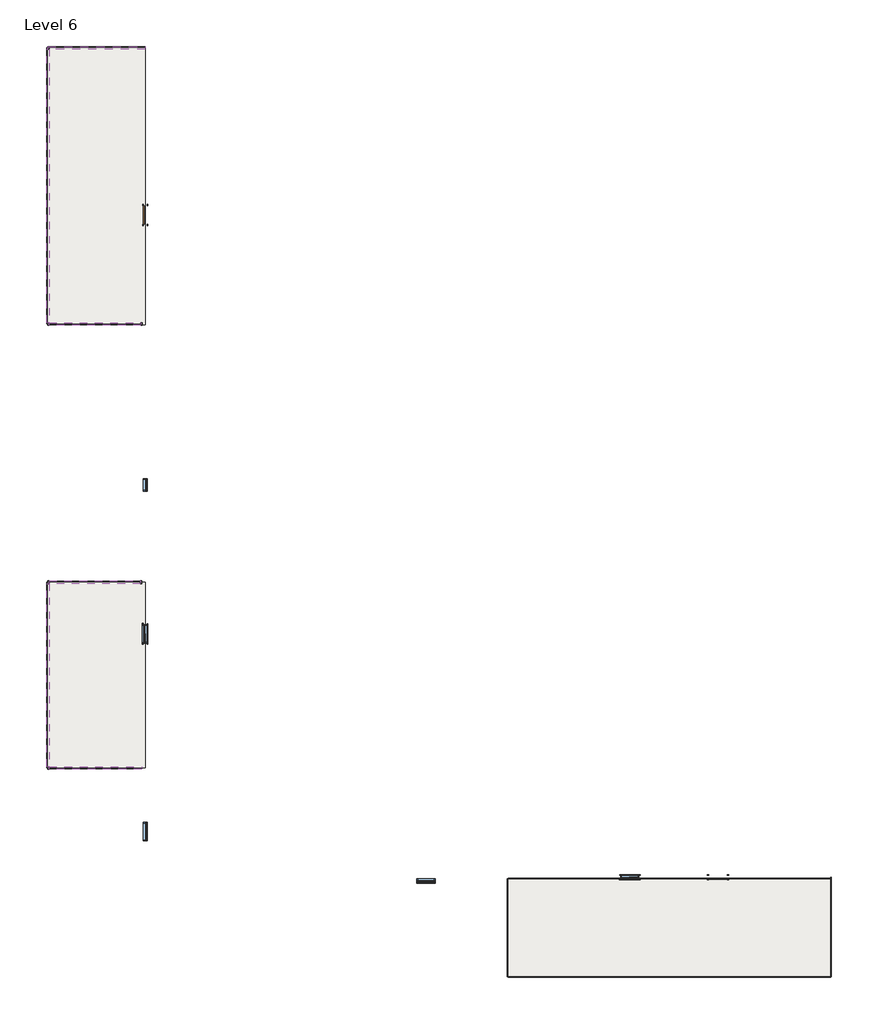
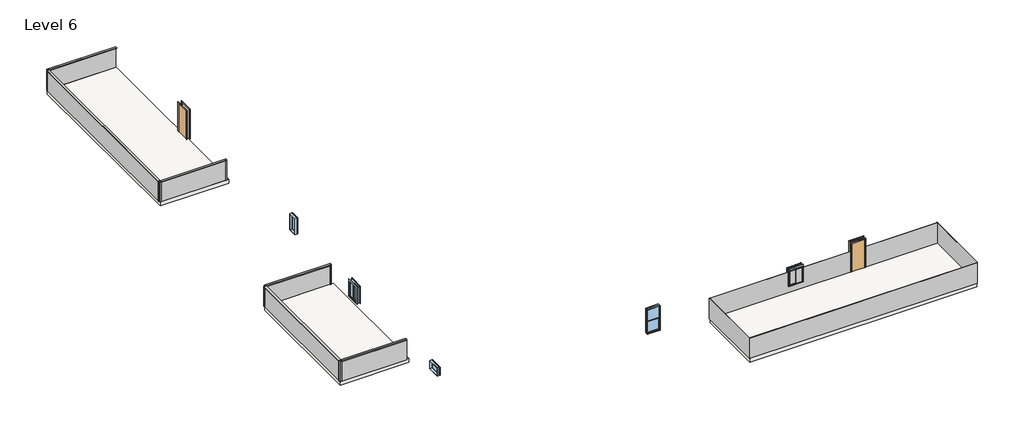
# One storey: 15 members, 10 plates, 5 windows, 3 slabs, 2 doors.
"""IFC4 building model written with IfcOpenShell, lengths in millimetres."""

from ifc_helpers import new_model, si_unit, frame, origin, place, context, project, spatial, polyline, outline, extrude, transform, mapped, element, save
from components import door_54dd4da4, door_719f80de, member_4491d118, member_b978f1c8, member_fc9bce7c, member_8787ee90, member_f500ba6f, member_67196db4, member_44cf4dfe, system_panel_glazed_dbf8c7ac, system_panel_glazed_64af9de3, system_panel_glazed_abcfc967, system_panel_glazed_6e908680, system_panel_glazed_242742f8, system_panel_glazed_fce9463a, system_panel_glazed_c13b8b16, system_panel_glazed_066de0f8, system_panel_glazed_7f285cc4, window_f274a882, window_80bd9af0, window_57c3ee1c, window_54100e87

model = new_model("IFC4")

# Units and contexts
model_context = context("Model", 3, world=origin())
ifc_project = project(units=[si_unit("LENGTHUNIT", "METRE", prefix="MILLI")], contexts=[model_context])

# Site, building, storey
site = spatial("IfcSite", under=ifc_project)
building = spatial("IfcBuilding", under=site)
storey = spatial("IfcBuildingStorey", under=building, Name="Level 6", Elevation=9753.6)

# Doors
placement = place(None, origin())
door_shape = door_54dd4da4(model_context)
element("IfcDoor", 1, ObjectType="Single-Flush : 36\" x 84\"", at=placement, inside=storey, context=model_context, shape_type="MappedRepresentation", body=[
    mapped(door_shape, transform((-15175.038074, 12428.2014639, 9753.6), x_axis=(0.0, 1.0, 0.0), y_axis=(-1.0, 0.0, 0.0), z_axis=(0.0, 0.0, 1.0))),
])
door_2_shape = door_719f80de(model_context)
element("IfcDoor", 2, ObjectType="Single-Flush : 36\" x 84\"", at=placement, inside=storey, context=model_context, shape_type="MappedRepresentation", body=[
    mapped(door_2_shape, transform((13526.961926, -20744.1985361, 9753.6), x_axis=(1.0, 0.0, 0.0), y_axis=(0.0, 1.0, 0.0), z_axis=(0.0, 0.0, 1.0))),
])

# Members
member_shape = member_4491d118(model_context)
element("IfcMember", 3, ObjectType="Rectangular Mullion : 2.5\" x 5\" rectangular", at=placement, inside=storey, context=model_context, shape_type="MappedRepresentation", body=[
    mapped(member_shape, transform((-20051.838074, 6979.9014639, 9753.6), x_axis=(-1.0, 0.0, 0.0), y_axis=(0.0, 1.0, 0.0), z_axis=(0.0, 0.0, -1.0))),
])
element("IfcMember", 4, ObjectType="Rectangular Mullion : 2.5\" x 5\" rectangular", at=placement, inside=storey, context=model_context, shape_type="MappedRepresentation", body=[
    mapped(member_shape, transform((-20051.838074, 20810.2014639, 9753.6), x_axis=(0.0, 1.0, 0.0), y_axis=(1.0, 0.0, 0.0), z_axis=(0.0, 0.0, -1.0))),
])
element("IfcMember", 5, ObjectType="Rectangular Mullion : 2.5\" x 5\" rectangular", at=placement, inside=storey, context=model_context, shape_type="MappedRepresentation", body=[
    mapped(member_shape, transform((-20051.838074, -5966.8213044, 9753.6), x_axis=(0.0, 1.0, 0.0), y_axis=(1.0, 0.0, 0.0), z_axis=(0.0, 0.0, -1.0))),
])
element("IfcMember", 6, ObjectType="Rectangular Mullion : 2.5\" x 5\" rectangular", at=placement, inside=storey, context=model_context, shape_type="MappedRepresentation", body=[
    mapped(member_shape, transform((-15357.6517659, -5966.8213044, 9753.6), x_axis=(1.0, 0.0, 0.0), y_axis=(0.0, -1.0, 0.0), z_axis=(0.0, 0.0, -1.0))),
])
element("IfcMember", 7, ObjectType="Rectangular Mullion : 2.5\" x 5\" rectangular", at=placement, inside=storey, context=model_context, shape_type="MappedRepresentation", body=[
    mapped(member_shape, transform((-20051.838074, -15263.2213044, 9753.6), x_axis=(-1.0, 0.0, 0.0), y_axis=(0.0, 1.0, 0.0), z_axis=(0.0, 0.0, -1.0))),
])
element("IfcMember", 8, ObjectType="Rectangular Mullion : 2.5\" x 5\" rectangular", at=placement, inside=storey, context=model_context, shape_type="MappedRepresentation", body=[
    mapped(member_shape, transform((-20051.838074, 6979.9014639, 11277.6), x_axis=(0.0, -1.0, 0.0), y_axis=(1.0, 0.0, 0.0), z_axis=(0.0, 0.0, 1.0))),
])
element("IfcMember", 9, ObjectType="Rectangular Mullion : 2.5\" x 5\" rectangular", at=placement, inside=storey, context=model_context, shape_type="MappedRepresentation", body=[
    mapped(member_shape, transform((-20051.838074, -5966.8213044, 11277.6), x_axis=(-1.0, 0.0, 0.0), y_axis=(0.0, -1.0, 0.0), z_axis=(0.0, 0.0, 1.0))),
])
element("IfcMember", 10, ObjectType="Rectangular Mullion : 2.5\" x 5\" rectangular", at=placement, inside=storey, context=model_context, shape_type="MappedRepresentation", body=[
    mapped(member_shape, transform((-20051.838074, -15263.2213044, 11277.6), x_axis=(0.0, -1.0, 0.0), y_axis=(1.0, 0.0, 0.0), z_axis=(0.0, 0.0, 1.0))),
])
element("IfcMember", 11, ObjectType="Rectangular Mullion : 2.5\" x 5\" rectangular", at=placement, inside=storey, context=model_context, shape_type="MappedRepresentation", body=[
    mapped(member_shape, transform((-15327.438074, 6979.9014639, 11277.6), x_axis=(1.0, 0.0, 0.0), y_axis=(0.0, 1.0, 0.0), z_axis=(0.0, 0.0, 1.0))),
])
member_2_shape = member_b978f1c8(model_context)
element("IfcMember", 12, ObjectType="Rectangular Mullion : 2.5\" x 5\" rectangular", at=placement, inside=storey, context=model_context, shape_type="MappedRepresentation", body=[
    mapped(member_2_shape, transform((-20051.838074, 20746.7014639, 11277.6), x_axis=(0.0, 0.0, 1.0), y_axis=(1.0, 0.0, 0.0), z_axis=(0.0, 1.0, 0.0))),
])
member_3_shape = member_fc9bce7c(model_context)
element("IfcMember", 13, ObjectType="Rectangular Mullion : 2.5\" x 5\" rectangular", at=placement, inside=storey, context=model_context, shape_type="MappedRepresentation", body=[
    mapped(member_3_shape, transform((-15175.038074, 20810.2014639, 11277.6), x_axis=(0.0, 0.0, 1.0), y_axis=(0.0, -1.0, 0.0), z_axis=(1.0, 0.0, 0.0))),
])
member_4_shape = member_8787ee90(model_context)
element("IfcMember", 14, ObjectType="Rectangular Mullion : 2.5\" x 5\" rectangular", at=placement, inside=storey, context=model_context, shape_type="MappedRepresentation", body=[
    mapped(member_4_shape, transform((-20051.838074, -6030.3213044, 11277.6), x_axis=(0.0, 0.0, 1.0), y_axis=(1.0, 0.0, 0.0), z_axis=(0.0, 1.0, 0.0))),
])
member_5_shape = member_f500ba6f(model_context)
element("IfcMember", 15, ObjectType="Rectangular Mullion : 2.5\" x 5\" rectangular", at=placement, inside=storey, context=model_context, shape_type="MappedRepresentation", body=[
    mapped(member_5_shape, transform((-15421.1517659, -5966.8213044, 11277.6), x_axis=(0.0, 0.0, 1.0), y_axis=(0.0, -1.0, 0.0), z_axis=(1.0, 0.0, 0.0))),
])
member_6_shape = member_67196db4(model_context)
element("IfcMember", 16, ObjectType="Rectangular Mullion : 2.5\" x 5\" rectangular", at=placement, inside=storey, context=model_context, shape_type="MappedRepresentation", body=[
    mapped(member_6_shape, transform((-19988.338074, -15263.2213044, 11277.6), x_axis=(0.0, 0.0, 1.0), y_axis=(0.0, 1.0, 0.0), z_axis=(-1.0, 0.0, 0.0))),
])
member_7_shape = member_44cf4dfe(model_context)
element("IfcMember", 17, ObjectType="Rectangular Mullion : 2.5\" x 5\" rectangular", at=placement, inside=storey, context=model_context, shape_type="MappedRepresentation", body=[
    mapped(member_7_shape, transform((-19988.338074, 6979.9014639, 11277.6), x_axis=(0.0, 0.0, 1.0), y_axis=(0.0, 1.0, 0.0), z_axis=(-1.0, 0.0, 0.0))),
])

# Plates
system_panel_glazed_shape = system_panel_glazed_dbf8c7ac(model_context)
element("IfcPlate", 18, ObjectType="System Panel : Glazed", at=placement, inside=storey, context=model_context, shape_type="MappedRepresentation", body=[
    mapped(system_panel_glazed_shape, transform((11088.561926, -20845.7985361, 9753.6), x_axis=(1.0, 0.0, 0.0), y_axis=(0.0, 1.0, 0.0), z_axis=(0.0, 0.0, 1.0))),
])
element("IfcPlate", 19, ObjectType="System Panel : Glazed", at=placement, inside=storey, context=model_context, shape_type="MappedRepresentation", body=[
    mapped(system_panel_glazed_shape, transform((11088.561926, -25722.5985361, 9753.6), x_axis=(-1.0, 0.0, 0.0), y_axis=(0.0, -1.0, 0.0), z_axis=(0.0, 0.0, 1.0))),
])
system_panel_glazed_2_shape = system_panel_glazed_64af9de3(model_context)
element("IfcPlate", 20, ObjectType="System Panel : Glazed", at=placement, inside=storey, context=model_context, shape_type="MappedRepresentation", body=[
    mapped(system_panel_glazed_2_shape, transform((19165.761926, -23233.3985361, 9753.6), x_axis=(0.0, -1.0, 0.0), y_axis=(1.0, 0.0, 0.0), z_axis=(0.0, 0.0, 1.0))),
])
system_panel_glazed_3_shape = system_panel_glazed_abcfc967(model_context)
element("IfcPlate", 21, ObjectType="System Panel : Glazed", at=placement, inside=storey, context=model_context, shape_type="MappedRepresentation", body=[
    mapped(system_panel_glazed_3_shape, transform((3011.361926, -23273.4060583, 9753.6), x_axis=(0.0, 1.0, 0.0), y_axis=(-1.0, 0.0, 0.0), z_axis=(0.0, 0.0, 1.0))),
])
system_panel_glazed_4_shape = system_panel_glazed_6e908680(model_context)
element("IfcPlate", 22, ObjectType="System Panel : Glazed", at=placement, inside=storey, context=model_context, shape_type="MappedRepresentation", body=[
    mapped(system_panel_glazed_4_shape, transform((-20051.838074, 13895.0514639, 9753.6), x_axis=(0.0, 1.0, 0.0), y_axis=(-1.0, 0.0, 0.0), z_axis=(0.0, 0.0, 1.0))),
])
system_panel_glazed_5_shape = system_panel_glazed_242742f8(model_context)
element("IfcPlate", 23, ObjectType="System Panel : Glazed", at=placement, inside=storey, context=model_context, shape_type="MappedRepresentation", body=[
    mapped(system_panel_glazed_5_shape, transform((-17613.438074, 20810.2014639, 9753.6), x_axis=(1.0, 0.0, 0.0), y_axis=(0.0, 1.0, 0.0), z_axis=(0.0, 0.0, 1.0))),
])
system_panel_glazed_6_shape = system_panel_glazed_fce9463a(model_context)
element("IfcPlate", 24, ObjectType="System Panel : Glazed", at=placement, inside=storey, context=model_context, shape_type="MappedRepresentation", body=[
    mapped(system_panel_glazed_6_shape, transform((-20051.838074, -10615.0213044, 9753.6), x_axis=(0.0, 1.0, 0.0), y_axis=(-1.0, 0.0, 0.0), z_axis=(0.0, 0.0, 1.0))),
])
system_panel_glazed_7_shape = system_panel_glazed_c13b8b16(model_context)
element("IfcPlate", 25, ObjectType="System Panel : Glazed", at=placement, inside=storey, context=model_context, shape_type="MappedRepresentation", body=[
    mapped(system_panel_glazed_7_shape, transform((-17704.7449199, -5966.8213044, 9753.6), x_axis=(1.0, 0.0, 0.0), y_axis=(0.0, 1.0, 0.0), z_axis=(0.0, 0.0, 1.0))),
])
system_panel_glazed_8_shape = system_panel_glazed_066de0f8(model_context)
element("IfcPlate", 26, ObjectType="System Panel : Glazed", at=placement, inside=storey, context=model_context, shape_type="MappedRepresentation", body=[
    mapped(system_panel_glazed_8_shape, transform((-17672.9949199, -15263.2213044, 9753.6), x_axis=(-1.0, 0.0, 0.0), y_axis=(0.0, -1.0, 0.0), z_axis=(0.0, 0.0, 1.0))),
])
system_panel_glazed_9_shape = system_panel_glazed_7f285cc4(model_context)
element("IfcPlate", 27, ObjectType="System Panel : Glazed", at=placement, inside=storey, context=model_context, shape_type="MappedRepresentation", body=[
    mapped(system_panel_glazed_9_shape, transform((-17689.638074, 6979.9014639, 9753.6), x_axis=(-1.0, 0.0, 0.0), y_axis=(0.0, -1.0, 0.0), z_axis=(0.0, 0.0, 1.0))),
])

# Slabs
element("IfcSlab", 28, ObjectType="Generic - 12\"", at=placement, inside=storey, context=model_context, shape_type="SweptSolid", body=[
    extrude(outline(polyline([(3011.361926, -20845.7985361), (19165.761926, -20845.7985361), (19165.761926, -25722.5985361), (3011.361926, -25722.5985361), (3011.361926, -20845.7985361)])), frame((0.0, 0.0, 9448.8), z_axis=(0.0, 0.0, 1.0), x_axis=(1.0, 0.0, 0.0)), (0.0, 0.0, 1.0), 304.8),
])
element("IfcSlab", 29, ObjectType="Generic - 12\"", at=placement, inside=storey, context=model_context, shape_type="SweptSolid", body=[
    extrude(outline(polyline([(-20051.838074, -15263.2213044), (-20051.838074, -5966.8213044), (-15175.038074, -5966.8213044), (-15175.038074, -15263.2213044), (-20051.838074, -15263.2213044)])), frame((0.0, 0.0, 9448.8), z_axis=(0.0, 0.0, 1.0), x_axis=(1.0, 0.0, 0.0)), (0.0, 0.0, 1.0), 304.8),
])
element("IfcSlab", 30, ObjectType="Generic - 12\"", at=placement, inside=storey, context=model_context, shape_type="SweptSolid", body=[
    extrude(outline(polyline([(-20051.838074, 20810.2014639), (-15175.038074, 20810.2014639), (-15175.038074, 6941.8014639), (-20051.838074, 6941.8014639), (-20051.838074, 20810.2014639)])), frame((0.0, 0.0, 9448.8), z_axis=(0.0, 0.0, 1.0), x_axis=(1.0, 0.0, 0.0)), (0.0, 0.0, 1.0), 304.8),
])

# Windows
window_shape = window_f274a882(model_context)
element("IfcWindow", 31, ObjectType="Double Hung : 36\" x 72\"", at=placement, inside=storey, context=model_context, shape_type="MappedRepresentation", body=[
    mapped(window_shape, transform((-1103.438074, -20921.9985361, 9997.4772003), x_axis=(-1.0, 0.0, 0.0), y_axis=(0.0, -1.0, 0.0), z_axis=(0.0, 0.0, 1.0))),
])
window_2_shape = window_80bd9af0(model_context)
element("IfcWindow", 32, ObjectType="Fixed : 24\" x 48\"", at=placement, inside=storey, context=model_context, shape_type="MappedRepresentation", body=[
    mapped(window_2_shape, transform((-15175.038074, -1128.1213044, 9753.6), x_axis=(0.0, -1.0, 0.0), y_axis=(1.0, 0.0, 0.0), z_axis=(0.0, 0.0, 1.0))),
])
window_3_shape = window_57c3ee1c(model_context)
element("IfcWindow", 33, ObjectType="Fixed : 36\" x 24\"", at=placement, inside=storey, context=model_context, shape_type="MappedRepresentation", body=[
    mapped(window_3_shape, transform((-15175.038074, -18496.2985361, 9753.6), x_axis=(0.0, -1.0, 0.0), y_axis=(1.0, 0.0, 0.0), z_axis=(0.0, 0.0, 1.0))),
])
window_4_shape = window_54100e87(model_context)
element("IfcWindow", 34, ObjectType="Slider with Trim : 36\" x 48\"", at=placement, inside=storey, context=model_context, shape_type="MappedRepresentation", body=[
    mapped(window_4_shape, transform((9107.361926, -20744.1985361, 9315.7942228), x_axis=(-1.0, 0.0, 0.0), y_axis=(0.0, -1.0, 0.0), z_axis=(0.0, 0.0, 1.0))),
])
element("IfcWindow", 35, ObjectType="Slider with Trim : 36\" x 48\"", at=placement, inside=storey, context=model_context, shape_type="MappedRepresentation", body=[
    mapped(window_4_shape, transform((-15175.038074, -8557.6213044, 9192.1414578), x_axis=(0.0, 1.0, 0.0), y_axis=(-1.0, 0.0, 0.0), z_axis=(0.0, 0.0, 1.0))),
])

save(model, "model.ifc")

# Revit data of these elements
# Type "Single-Flush : 36\" x 84\""
#   Type Mark = "1"
#   Construction Type Id = "MDOOR"
#   Assembly Code = "C1020"
#   Analytic Construction = "Metal"
#   Thickness = 0' - 2"
#   Heat Transfer Coefficient (U) = 0.651978 BTU/(h·ft²·°F)
#   Height = 7' - 0"
#   Trim Projection Ext = 0' - 1"
#   Trim Projection Int = 0' - 1"
#   Trim Width = 0' - 3"
#   Width = 3' - 0"
#   Define Thermal Properties by = 1
#   Door Material = Door - Panel
#   Frame Material = Door - Frame
#   Visual Light Transmittance = 0
#   Solar Heat Gain Coefficient = 0
#   Function = (empty or 0)
#   Wall Closure = (empty or 0)
# Type "Rectangular Mullion : 2.5\" x 5\" rectangular"
#   built-in parameter 1007304 = 0.416667 (stored number, unit not read)
#   built-in parameter 1007301 = 0.104167 (stored number, unit not read)
#   built-in parameter 1007300 = 0.104167 (stored number, unit not read)
# Type "System Panel : Glazed"
#   Construction Type Id = "GSP4R"
#   Analytic Construction = "1/8 in Pilkington single glazing"
#   Visual Light Transmittance = 0.9
#   Solar Heat Gain Coefficient = 0.86
#   Heat Transfer Coefficient (U) = 1.18115 BTU/(h·ft²·°F)
# Type "Generic - 12\""
#   Assembly Code = "B1010"
#   Function = 0
#   Layers, outside or top first: 1' - 0" no material (function 1)
# Type "Double Hung : 36\" x 72\""
#   Type Mark = "18"
#   Construction Type Id = "GSP4R"
#   Assembly Code = "B2020100"
#   Analytic Construction = "1/8 in Pilkington single glazing"
#   Visual Light Transmittance = 0.9
#   Solar Heat Gain Coefficient = 0.78
#   Heat Transfer Coefficient (U) = 0.6496 BTU/(h·ft²·°F)
#   Height = 6' - 0"
#   Default Sill Height = 1' - 0"
#   Width = 3' - 0"
#   Window Inset = 0' - 0 3/4"
#   Define Thermal Properties by = 1
#   Glass Pane Material = Glass
#   Sash Material = Sash
#   Description = (empty or 0)
#   Wall Closure = (empty or 0)
# Type "Fixed : 24\" x 48\""
#   Type Mark = "2"
#   Construction Type Id = "GSP4R"
#   Assembly Code = "B2020100"
#   Analytic Construction = "1/8 in Pilkington single glazing"
#   Visual Light Transmittance = 0.9
#   Solar Heat Gain Coefficient = 0.78
#   Heat Transfer Coefficient (U) = 0.6496 BTU/(h·ft²·°F)
#   Height = 4' - 0"
#   Default Sill Height = 3' - 0"
#   Width = 2' - 0"
#   Window Inset = 0' - 0 3/4"
#   Define Thermal Properties by = 1
#   Glass Pane Material = Glass
#   Sash Material = Sash
#   Wall Closure = (empty or 0)
# Type "Fixed : 36\" x 24\""
#   Type Mark = "8"
#   Construction Type Id = "GSP4R"
#   Assembly Code = "B2020100"
#   Analytic Construction = "1/8 in Pilkington single glazing"
#   Visual Light Transmittance = 0.9
#   Solar Heat Gain Coefficient = 0.78
#   Heat Transfer Coefficient (U) = 0.6496 BTU/(h·ft²·°F)
#   Height = 2' - 0"
#   Default Sill Height = 3' - 0"
#   Width = 3' - 0"
#   Window Inset = 0' - 0 3/4"
#   Define Thermal Properties by = 1
#   Glass Pane Material = Glass
#   Sash Material = Sash
#   Wall Closure = (empty or 0)
# Type "Slider with Trim : 36\" x 48\""
#   Type Mark = "22"
#   Construction Type Id = "GSP4R"
#   Assembly Code = "B2020100"
#   Analytic Construction = "1/8 in Pilkington single glazing"
#   Visual Light Transmittance = 0.9
#   Solar Heat Gain Coefficient = 0.78
#   Heat Transfer Coefficient (U) = 0.6496 BTU/(h·ft²·°F)
#   Height = 4' - 0"
#   Default Sill Height = 3' - 0"
#   Trim Projection - Ext. = 0' - 0 3/4"
#   Trim Projection - Int. = 0' - 0 3/4"
#   Trim Width - Exterior = 0' - 3 1/2"
#   Trim Width - Interior = 0' - 3 1/2"
#   Width = 3' - 0"
#   Window Inset = 0' - 0 3/4"
#   Define Thermal Properties by = 1
#   Glass Pane Material = Glass
#   Sash Material = Sash
#   Trim Exterior Material = Trim
#   Trim Interior Material = Trim
#   Wall Closure = (empty or 0)
# Elements 1, 2 (IfcDoor, "Single-Flush : 36\" x 84\"")
#   Phase Created = New Construction
#   Materials on its faces: "Door - Frame", "Door - Panel"
# Elements 3, 4, 5, 6, 7, 8, 9, 10, 11, 12, 13, 14, 15, 16, 17 (IfcMember, "Rectangular Mullion : 2.5\" x 5\" rectangular")
#   Phase Created = New Construction
#   Materials on its faces: "Aluminum"
# Elements 18, 19, 20, 21, 22, 23, 24, 25, 26, 27 (IfcPlate, "System Panel : Glazed")
#   Phase Created = New Construction
#   Materials on its faces: "Glass"
# Elements 28, 29, 30 (IfcSlab, "Generic - 12\"")
#   built-in parameter 1001955 = 3.14159 (stored number, unit not read)
#   Height Offset From Level = 0' - 0"
#   Phase Created = New Construction
#   Materials on its faces: "Default Floor"
# Element 31 (IfcWindow, "Double Hung : 36\" x 72\"")
#   Mark = "9"
#   Phase Created = New Construction
#   Materials on its faces: "Sash", "Glass"
# Element 32 (IfcWindow, "Fixed : 24\" x 48\"")
#   Mark = "53"
#   Phase Created = New Construction
#   Materials on its faces: "Sash", "Glass"
# Element 33 (IfcWindow, "Fixed : 36\" x 24\"")
#   Mark = "75"
#   Phase Created = New Construction
#   Materials on its faces: "Sash", "Glass"
# Element 34 (IfcWindow, "Slider with Trim : 36\" x 48\"")
#   Mark = "31"
#   Phase Created = New Construction
#   Materials on its faces: "Sash", "Trim", "Glass"
# Element 35 (IfcWindow, "Slider with Trim : 36\" x 48\"")
#   Mark = "42"
#   Phase Created = New Construction
#   Materials on its faces: "Sash", "Trim", "Glass"
# Materials
#   "Door - Panel": class "Wood", colour RGB 210 159 95, transparency 0
#   "Door - Frame": colour RGB 118 70 51, transparency 0
#   "Glass": class "Glass", colour RGB 0 128 192, transparency 0.75, Description = "Soda Lime Glass", Cost = 0
#   "Sash": class "Wood", colour RGB 224 178 126, transparency 0
#   "Trim": class "Wood", colour RGB 224 178 126, transparency 0
#   "Aluminum": class "Metal", colour RGB 247 247 247, transparency 0, Description = "Aluminum 6061", Cost = 0
#   "Default Floor": colour RGB 128 128 128, transparency 0
